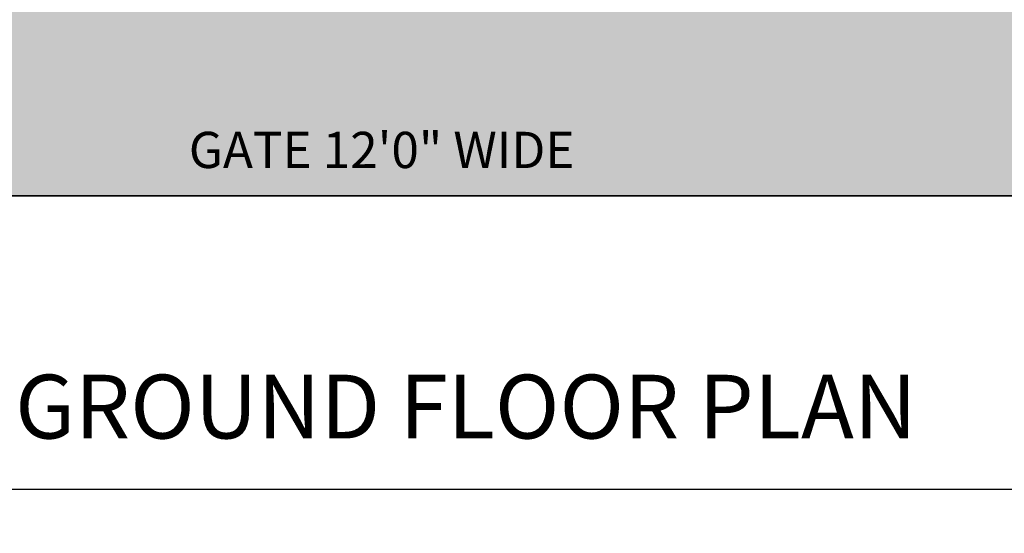
# Model space of a CAD drawing. Units: inches. Extents: x 389 to 971, y 148 to 870.
# Tile 1 of 14: x 448 to 565, y 194 to 256. Entities that reach past the tile are written whole.
import ezdxf

# ---------------------------------------------------------------- set-up
doc = ezdxf.new("R2010")
doc.units = ezdxf.units.IN
doc.header["$MEASUREMENT"] = 0
for name, color, linetype, lineweight in [('A-ANNO-DIMS', 2, 'Continuous', 18), ('A-ANNO-TEXT', 7, 'Continuous', 18), ('A-ANNO-TITL', 7, 'Continuous', 25), ('C-PROP', 7, 'Continuous', 35), ('L-GATE', 4, 'Continuous', 25), ('L-GRND-BASE-PATT', 8, 'Continuous', 13)]:
    doc.layers.add(name, color=color, linetype=linetype, lineweight=lineweight)
doc.layers.add('L-GRND-PATT', color=39, linetype='Continuous', lineweight=13, true_color=0x603913)
doc.styles.get("Standard").update_dxf_attribs({"font": 'arial.ttf'})
doc.dimstyles.get("Standard").update_dxf_attribs({"dimtxt": 8, "dimasz": 8, "dimexe": 0.18, "dimexo": 0.0625, "dimgap": 0.09, "dimtad": 0, "dimtih": 1, "dimtoh": 1, "dimdec": 0, "dimzin": 0, "dimdsep": 46, "dimlunit": 3, "dimtxsty": 'Standard', "dimcen": 0.09, "dimadec": 0, "dimazin": 0, "dimtfac": 1, "dimtdec": 0, "dimtofl": 0, "dimtmove": 0, "dimatfit": 3, "dimfxl": 1, "dimtolj": 1, "dimtzin": 0, "dimarcsym": 0})

# ---------------------------------------------------------------- blocks, each defined once
blk = doc.blocks.new('*D44')
at = {"layer": 'A-ANNO-DIMS', "color": 0, "lineweight": -2, "transparency": 16777216}
for p, q in [((428.216024, 234.582013), (428.216024, 199.495293)), ((848.2160239999998, 234.582013), (848.2160239999998, 199.495293)), ((436.216024, 199.675293), (629.1410308212824, 199.675293)), ((840.2160239999998, 199.675293), (647.2910171787175, 199.675293))]:
    blk.add_line(p, q, dxfattribs=at)
at = {"layer": 'A-ANNO-DIMS', "color": 0, "transparency": 16777216}
for points in [[(436.216024, 201.0086263333334), (436.216024, 198.3419596666666), (428.216024, 199.675293)], [(840.2160239999998, 201.0086263333334), (840.2160239999998, 198.3419596666666), (848.2160239999998, 199.675293)]]:
    blk.add_solid(points, dxfattribs=at)
at = {"layer": 'Defpoints', "color": 0, "transparency": 16777216}
for p in [(428.216024, 234.644513), (848.2160239999998, 234.644513), (848.2160239999998, 199.675293)]:
    blk.add_point(p, dxfattribs=at)
at = {"layer": 'A-ANNO-DIMS', "color": 0, "transparency": 16777216, "insert": (638.216024, 199.675293), "char_height": 8, "attachment_point": 5}
blk.add_mtext('\\A1;420', dxfattribs=at)

msp = doc.modelspace()

# ---------------------------------------------------------------- hatches: boundary and pattern name
at = {"layer": 'L-GRND-BASE-PATT'}
h = msp.add_hatch(color=256, dxfattribs=at)
h.dxf.hatch_style = 1
edge = h.paths.add_edge_path(flags=16)
edge.add_ellipse((8782.002602781105, 354.2472542798386), major_axis=(-8296.949265805946, 5.39345e-11), ratio=0.8423038695428886, start_angle=-0.0902290885933894, end_angle=0.3838667787920258, ccw=False)
edge.add_ellipse((485.0533369751568, 368.2895347624687), major_axis=(-1.159084047334488, 1.838e-13), ratio=0.8423038695439892, start_angle=9.094947017729282e-12, end_angle=90.00000000000898, ccw=False)
edge.add_line((483.8942529278224, 368.2895347624687), (483.8942529278225, 387.6039063360424))
edge.add_ellipse((485.0533369751571, 387.2465553762829), major_axis=(1.159084047334488, 1.838e-13), ratio=0.8423038695439892, start_angle=89.99999999999102, end_angle=179.9999999999909, ccw=False)
edge.add_line((485.0533369751572, 388.2228563544795), (485.5047440247956, 388.2228563544795))
edge.add_ellipse((898.8202485054873, 372.489720535918), major_axis=(413.7373561031672, 1.26113e-11), ratio=0.8423038695441164, start_angle=176.3495724142986, end_angle=177.8200496863524, ccw=False)
edge.add_ellipse((535.9119176052733, 196.3854951855018), major_axis=(-245.3971626940985, 1.013648e-10), ratio=0.8423038695442548, start_angle=-77.87403444769302, end_angle=-76.2194710104792, ccw=False)
edge.add_ellipse((535.9119176052684, 201.7546502845751), major_axis=(239.1273775699096, 1.008988e-10), ratio=0.842303869543627, start_angle=100.20953899711827, end_angle=102.44462729341922, ccw=False)
edge.add_ellipse((473.3138688667988, 564.9222417143382), major_axis=(196.5636751472093, 8.4793e-12), ratio=0.8423038695439335, start_angle=-80.74343399280163, end_angle=-77.44506735586587)
edge.add_line((509.5535496243029, 402.1940957519602), (514.3535105156315, 404.8483349684994))
edge.add_line((514.3535105156315, 404.8483349684994), (514.3535105156315, 404.7971763262221))
edge.add_ellipse((514.3535105156316, 404.2643898676136), major_axis=(0.5795420236673633, 2e-16), ratio=0.8423038695437671, start_angle=52.06686954015339, end_angle=90.00000000001342, ccw=False)
edge.add_line((514.671564037824, 404.672460591463), (519.1534714069603, 402.19409575196))
edge.add_ellipse((555.3931521644682, 564.9222417143374), major_axis=(-196.5636751472384, 3.62381e-11), ratio=0.8423038695438114, start_angle=77.44506735587258, end_angle=80.74343399280833)
edge.add_ellipse((492.795103425985, 201.7546502845724), major_axis=(239.12737756976, 4.82267e-11), ratio=0.8423038695441539, start_angle=77.55537270654253, end_angle=79.7904610028433, ccw=False)
edge.add_ellipse((492.7951034259847, 196.3854951855023), major_axis=(245.3971626940514, 1.422861e-10), ratio=0.8423038695444116, start_angle=76.21947101046823, end_angle=77.87403444768199, ccw=False)
edge.add_ellipse((129.8867725257751, 372.4897205359271), major_axis=(-413.7373561031673, 2.44623e-11), ratio=0.8423038695441432, start_angle=182.179950313648, end_angle=183.6504275857018, ccw=False)
edge.add_line((543.2022770064673, 388.2228563544788), (544.0779382625514, 388.2228563544787))
edge.add_ellipse((543.6536840561057, 387.2465553762822), major_axis=(-1.159084047334545, 1.527e-13), ratio=0.8423038695438989, start_angle=180.0000000000075, end_angle=270.00000000000756, ccw=False)
edge.add_line((544.8127681034401, 387.2465553762826), (544.8127681034399, 367.9321838027083))
edge.add_ellipse((543.6536840561054, 368.2895347624679), major_axis=(1.159084047334544, 7.24e-14), ratio=0.8423038695439478, start_angle=269.9999999999964, end_angle=359.9999999999964, ccw=False)
edge.add_ellipse((-7753.295581726658, 354.2472542799028), major_axis=(-8296.949265782761, 2.068448e-10), ratio=0.8423038695442414, start_angle=179.6161332212083, end_angle=180.0902290885951, ccw=False)
edge.add_line((543.3912265319653, 298.6607849184036), (544.0779382625504, 298.6607849184036))
edge.add_ellipse((543.6536840561046, 297.6844839402071), major_axis=(1.159084047334431, 1.769e-13), ratio=0.8423038695439814, start_angle=-1.1482370609883219e-11, end_angle=89.99999999999119, ccw=False)
edge.add_line((544.8127681034391, 297.684483940207), (544.8127681034387, 278.3701123666333))
edge.add_ellipse((543.6536840561043, 278.727463326393), major_axis=(-1.159084047334431, 2.574e-13), ratio=0.8423038695440306, start_angle=90.00000000001268, end_angle=180.0000000000099, ccw=False)
edge.add_line((543.6536840561045, 277.7511623481965), (543.1566278692261, 277.7511623481965))
edge.add_ellipse((-7753.295581726658, 354.2472542799028), major_axis=(-8296.949265782761, 2.068448e-10), ratio=0.8423038695442414, start_angle=179.3813568036816, end_angle=179.4717285281829, ccw=False)
edge.add_ellipse((542.4236240941387, 263.2762864208561), major_axis=(-1.738626071001761, 2.132e-13), ratio=0.8423038695439151, start_angle=179.3717627838137, end_angle=248.464756601011, ccw=False)
edge.add_ellipse((-7753.875123750511, 354.2472542780016), major_axis=(-8298.740341433751, 2.4782644722e-06), ratio=0.8423038662721074, start_angle=179.3534459200609, end_angle=179.3717628008941, ccw=False)
edge.add_ellipse((540.0116322079951, 260.6509346628677), major_axis=(-4.109243751168186, 2.384e-13), ratio=0.842303869543976, start_angle=90.0000000000635, end_angle=179.3534459029233, ccw=False)
edge.add_line((540.0116322079991, 257.1897027503593), (488.6953888232593, 257.1897027503609))
edge.add_ellipse((488.6953888232669, 260.6509346628715), major_axis=(4.10924375117072, 1.262e-13), ratio=0.8423038695439824, start_angle=180.6465540970565, end_angle=269.9999999998589, ccw=False)
edge.add_ellipse((8782.582144816053, 354.2472542821698), major_axis=(-8298.740341477976, 1.8591886369e-06), ratio=0.8423038720186145, start_angle=0.6282372290784792, end_angle=0.6465541099116194, ccw=False)
edge.add_ellipse((486.2833969371199, 263.2762864208594), major_axis=(-1.738626071002378, 2.7e-13), ratio=0.8423038695439394, start_angle=-68.46475649596817, end_angle=0.6282372161796275, ccw=False)
edge.add_ellipse((8782.002602781105, 354.2472542798386), major_axis=(-8296.949265805946, 5.39345e-11), ratio=0.8423038695428886, start_angle=0.5282714718171064, end_angle=0.6465540970606867, ccw=False)
edge.add_line((485.5503931620382, 277.7511623481972), (484.6290827687102, 277.7511623481972))
edge.add_ellipse((485.0533369751559, 278.7274633263938), major_axis=(-1.159084047334545, 3.11e-13), ratio=0.8423038695439968, start_angle=1.5404566511278972e-11, end_angle=90.000000000012, ccw=False)
edge.add_line((483.8942529278214, 278.7274633263938), (483.8942529278216, 298.0418348999672))
edge.add_ellipse((485.053336975156, 297.6844839402078), major_axis=(1.159084047334488, 1.025e-13), ratio=0.8423038695440382, start_angle=89.99999999999488, end_angle=179.9999999999949, ccw=False)
edge = h.paths.add_edge_path(flags=0)
edge.add_ellipse((8782.002602781096, 354.247254279773), major_axis=(-8295.790181758603, 9.87839e-10), ratio=0.8423038695486498, start_angle=0.05559431350519617, end_angle=0.37776419391582294, ccw=False)
edge.add_line((486.2179253655185, 346.1978202249628), (489.3905023836935, 335.8383575186984))
edge.add_ellipse((3386.011413077446, 329.726312794031), major_axis=(-2896.629999631248, 1.069454e-10), ratio=0.8423038695494893, start_angle=-0.1208973690315206, end_angle=0.3640763488915184)
edge.add_line((489.4638383140943, 311.3204429697198), (486.4665645878948, 299.5520931219791))
edge = h.paths.add_edge_path(flags=0)
edge.add_ellipse((514.3535105156315, 391.3730654902235), major_axis=(-115.1512533244504, 1.8736e-12), ratio=0.8423038695439684, start_angle=76.4018653097696, end_angle=103.5981346902308)
edge.add_line((537.3427693057832, 296.3333211885938), (537.342769305783, 281.5897392316151))
edge.add_ellipse((514.3535105156313, 376.6294835332447), major_axis=(-115.1512533244486, 9.02e-13), ratio=0.8423038695439828, start_angle=76.40186530976922, end_angle=103.59813469023032, ccw=False)
edge.add_line((491.3642517254773, 281.5897392316156), (491.3642517254774, 296.3333211885945))
edge = h.paths.add_edge_path(flags=0)
edge.add_line((491.3642517254777, 337.0752369161334), (489.6529508739416, 349.9015767089268))
edge.add_ellipse((510.1338164488795, 298.7862183048575), major_axis=(64.04807894948699, 3.9006e-12), ratio=0.8423038695439252, start_angle=94.27742096304979, end_angle=111.83495379670401, ccw=False)
edge.add_line((506.106812905481, 352.6274231954524), (522.600208125781, 352.6274231954521))
edge.add_ellipse((518.5732045823798, 298.7862183048586), major_axis=(64.04807894948067, 3.24e-14), ratio=0.8423038695439885, start_angle=68.16504620328948, end_angle=85.72257903694378, ccw=False)
edge.add_line((539.05407015732, 349.9015767089259), (537.3427693057835, 337.0752369161327))
edge.add_ellipse((516.5461636849332, 287.5825181681899), major_axis=(62.33048198262021, 1.5954e-12), ratio=0.8423038695439995, start_angle=67.20808512240782, end_angle=85.12993040286212)
edge.add_line((521.0080028322477, 339.9490379899644), (507.6990181990146, 339.9490379899646))
edge.add_ellipse((512.1608573463288, 287.5825181681774), major_axis=(62.33048198263887, 2.0798e-12), ratio=0.8423038695439498, start_angle=94.8700695971331, end_angle=112.791914877584)
edge = h.paths.add_edge_path(flags=0)
edge.add_ellipse((493.6824198201462, 273.9438556676354), major_axis=(-2.318168094668919, 1.896e-13), ratio=0.8423038695439611, start_angle=-89.99999999999523, end_angle=4.718003765447065e-12, ccw=False)
edge.add_line((493.6824198201462, 275.8964576240284), (535.3743409680425, 275.8964576240277))
edge.add_ellipse((535.024601211114, 273.9438556676347), major_axis=(2.318168094668976, 2.946e-13), ratio=0.8423038695439647, start_angle=-7.275957614183426e-12, end_angle=89.99999999998943, ccw=False)
edge.add_line((537.342769305783, 273.9438556676347), (537.3427693057827, 258.698332706474))
edge.add_line((537.3427693057827, 258.698332706474), (540.5911742316662, 258.6983327064739))
edge.add_ellipse((540.5911742316634, 260.6509346628669), major_axis=(-2.318168094668839, 2.143e-13), ratio=0.8423038695440144, start_angle=90.00000000008203, end_angle=179.3534459029346)
edge.add_line((540.5911742316662, 258.6983327064739), (487.7691399811528, 258.6983327064755))
edge.add_ellipse((488.1158467995968, 260.6509346628684), major_axis=(2.318168094668909, 7.48e-14), ratio=0.8423038695439647, start_angle=180.6465540970884, end_angle=269.9999999999081)
edge.add_line((488.1158467995931, 258.6983327064755), (491.3642517254771, 258.6983327064754))
edge.add_line((491.3642517254771, 258.6983327064754), (491.3642517254771, 274.2384428182294))
h.paths.add_polyline_path([(746.1375687288224, 327.3223047166553), (750.1400147212453, 327.3223047166553), (750.1400147212453, 326.2830696147227), (798.1693712998389, 326.2830696147227), (798.1693712998389, 327.3223047166553), (802.1718172922616, 327.3223047166553), (802.1718172922616, 309.9783792024682, -0.1904762075443491), (746.1375687288224, 309.9783668090107)], flags=16)
h.paths.add_polyline_path([(782.1595875801748, 313.5684994305933), (782.1595893317732, 309.0414930416419, -0.0496282101666581), (766.1497986905329, 309.0414910503953), (766.1498004421323, 313.5684994305933)], flags=0)
h.paths.add_polyline_path([(755.1858908233534, 344.9352232902417), (755.1858908233534, 373.916311072083), (788.1243995226009, 373.916311072083), (788.1243995226009, 344.9352232902417)], flags=16)
h.paths.add_polyline_path([(757.1858908233535, 346.9352232902417), (757.1858908233535, 371.916311072083), (786.1243995226009, 371.916311072083), (786.1243995226009, 346.9352232902417)], flags=0)
h.paths.add_polyline_path([(803.6445810111745, 338.4878931208803), (803.6445810111745, 342.4903391133031), (804.6838161131072, 342.4903391133031), (804.6838161131072, 390.5196956918968), (803.6445810111748, 390.5196956918968), (803.6445810111748, 394.5221416843196), (820.9885065253617, 394.5221416843196, -0.1904762075443491), (820.9885189188192, 338.4878931208803)], flags=16)
h.paths.add_polyline_path([(806.8706930931005, 326.6963103558256), (806.4254411777042, 327.1415622712219), (806.4723791864895, 326.6297175483474)], flags=16)
h.paths.add_polyline_path([(822.0328146004263, 317.4007976138144), (822.1941503181826, 317.8932883068639), (821.562628166435, 317.9885306563034)], flags=16)
h.paths.add_polyline_path([(817.3983862972365, 358.5001248341902), (817.3983862972365, 374.5099119722327), (821.9253926861879, 374.5099137238312, -0.049628210166658), (821.9253946774346, 358.5001230825909)], flags=0)
h.paths.add_polyline_path([(808.1446344648577, 418.9736619306146), (808.2246858861593, 418.5632188717996), (808.5395491501399, 418.5787472453325)], flags=16)
h.paths.add_polyline_path([(820.3158762739024, 412.6690288868844), (820.4772119916585, 413.161519579934), (819.8456898399113, 413.2567619293735)], flags=16)
h.paths.add_polyline_path([(466.3155093563569, 235.5246322146605), (517.3806533266912, 235.5246322146605), (517.3806533266912, 244.4269231682286), (466.3155093563569, 244.4269231682286)], flags=24)
h.paths.add_polyline_path([(739.8737195480014, 256.2000079819968), (815.4040239338423, 256.2000079819968), (815.4040239338423, 265.3453807094367), (739.8737195480014, 265.3453807094367)], flags=24)
h.paths.add_polyline_path([(750.6081538187397, 393.6666679930368), (791.5680640722773, 393.6666679930368), (791.5680640722773, 412.3933175868746), (750.6081538187397, 412.3933175868746)], flags=24)
h.paths.add_polyline_path([(438.9630812812552, 410.0618566955462), (484.6203810968238, 410.0618566955462), (484.6203810968238, 429.1217352891893), (438.9630812812552, 429.1217352891893)], flags=24)
edge = h.paths.add_edge_path()
edge.add_line((839.2160244416713, 285.6445131961097), (611.8786784019748, 285.6445131961099))
edge.add_line((611.8786784019748, 285.6445131961099), (604.3870116090119, 285.6445131961097))
edge.add_line((604.3870116090119, 285.6445131961097), (595.3870116090119, 285.6445131961097))
edge.add_line((595.3870116090119, 285.6445131961097), (595.3870116090118, 370.1553848722774))
edge.add_line((595.3870116090118, 370.1553848722774), (604.0816928471932, 370.1553848722774))
edge.add_line((604.0816928471932, 370.1553848722774), (604.0816928471932, 371.3788335667469))
edge.add_line((604.0816928471932, 371.3788335667469), (632.0194586761203, 371.3788335667469))
edge.add_arc((604.0816928471932, 370.1553848722773), 27.96454158787471, 2.507490703587644, 90.00000000000003)
edge.add_line((604.0816928471932, 398.1199264601519), (599.8870116090108, 398.1652144688576))
edge.add_line((599.8870116090108, 398.1652144688576), (604.4225424425357, 398.1652144688576))
edge.add_arc((604.4225424425357, 428.4020866923496), 30.23687222349201, 270.0000000000002, 357.492509296413)
edge.add_line((634.6304631740308, 427.0792235325719), (604.4225424425357, 427.0792235325719))
edge.add_line((604.4225424425357, 427.0792235325719), (604.4225424425357, 428.4020866923497))
edge.add_line((604.4225424425357, 428.4020866923497), (599.8870116090119, 428.4020866923497))
edge.add_line((599.8870116090119, 428.4020866923497), (595.3870116090116, 428.4020866923497))
edge.add_line((595.3870116090116, 428.4020866923497), (595.3870116090118, 434.6445131961097))
edge.add_line((595.3870116090118, 434.6445131961097), (585.0790669792458, 434.6445131961097))
edge.add_line((585.0790669792458, 434.6445131961097), (540.3921730610418, 434.6445131961097))
edge.add_line((540.3921730610418, 434.6445131961097), (526.712508448134, 434.6445131961097))
edge.add_line((526.712508448134, 434.6445131961097), (488.4094553949635, 434.6445131961097))
edge.add_line((488.4094553949635, 434.6445131961097), (432.2160244416713, 434.6445131961097))
edge.add_line((432.2160244416713, 434.6445131961097), (432.2160244416713, 243.6445131961098))
edge.add_line((432.2160244416713, 243.6445131961098), (437.2160244416714, 243.6445131961098))
edge.add_line((437.2160244416714, 243.6445131961098), (437.2160244416714, 234.6445131961098))
edge.add_line((437.2160244416714, 234.6445131961098), (581.2160244416713, 234.6445131961098))
edge.add_line((581.2160244416713, 234.6445131961098), (581.2160244416713, 238.6445131961097))
edge.add_line((581.2160244416713, 238.6445131961097), (581.2160244416713, 243.6445131961098))
edge.add_line((581.2160244416713, 243.6445131961098), (590.2160244416713, 243.6445131961098))
edge.add_line((590.2160244416713, 243.6445131961098), (590.2160244416713, 238.6445131961097))
edge.add_line((590.2160244416713, 238.6445131961097), (839.2160244416713, 238.6445131961098))
edge.add_line((839.2160244416713, 238.6445131961098), (839.2160244416713, 285.6445131961097))
at = {"layer": 'L-GRND-PATT'}
h = msp.add_hatch(dxfattribs=at)
h.set_pattern_fill('EARTH', color=256, angle=45)
h.set_pattern_definition([(45, (0, 0), (0, 8.980256121069154), [6.349999999999999, -6.349999999999999]), (45, (-1.683798022700466, 1.683798022700466), (0, 8.980256121069154), [6.349999999999999, -6.349999999999999]), (45, (-3.367596045400933, 3.367596045400933), (0, 8.980256121069154), [6.349999999999999, -6.349999999999999]), (135, (-3.367596045400933, 4.490128060534576), (-8.980256121069154, 0), [6.349999999999999, -6.349999999999999]), (135, (-1.683798022700466, 6.173926083235043), (-8.980256121069154, 0), [6.349999999999999, -6.349999999999999]), (135, (0, 7.85772410593551), (-8.980256121069154, 0), [6.349999999999999, -6.349999999999999])])
h.paths.add_polyline_path([(432.2160244416713, 243.6445131961098), (437.2160244416714, 243.6445131961098), (437.2160244416714, 234.6445131961098), (581.2160244416713, 234.6445131961098), (581.2160244416713, 238.6445131961097), (581.2160244416713, 243.6445131961098), (590.2160244416713, 243.6445131961098), (590.2160244416713, 238.6445131961097), (839.2160244416713, 238.6445131961098), (839.2160244416712, 285.6445131961097), (810.0513609197296, 285.6445131961097), (733.8056934525983, 285.6445131961099), (684.2433676403508, 285.6445131961098), (611.8786784019748, 285.6445131961099), (604.3870116090119, 285.6445131961097), (595.3870116090119, 285.6445131961097), (595.3870116090118, 370.1553848722774), (604.0816928471932, 370.1553848722774), (604.0816928471932, 371.3788335667469), (632.0194586761203, 371.3788335667469, 0.4014527144963568), (604.0816928471932, 398.119926460152), (599.8870116090127, 398.1652144688576), (604.4225424425357, 398.1652144688576, 0.4014527144963579), (634.6304631740308, 427.0792235325719), (604.4225424425357, 427.0792235325719), (604.4225424425357, 428.4020866923497), (599.8870116090119, 428.4020866923497), (595.3870116090116, 428.4020866923497), (595.3870116090118, 434.6445131961097), (585.0790669792458, 434.6445131961097), (540.3921730610418, 434.6445131961097), (526.712508448134, 434.6445131961097), (488.4094553949635, 434.6445131961097), (432.2160244416713, 434.6445131961097)])
edge = h.paths.add_edge_path(flags=16)
edge.add_line((483.8942529278214, 278.7274633263938), (483.8942529278216, 298.2563878122772))
edge.add_ellipse((485.053336975156, 297.6844839402078), major_axis=(1.159084047334488, 1.025e-13), ratio=0.8423038695440382, start_angle=89.99999999999488, end_angle=179.9999999999949, ccw=False)
edge.add_ellipse((8782.002602781105, 354.2472542798386), major_axis=(-8296.949265805946, 5.39345e-11), ratio=0.8423038695428886, start_angle=-0.0902290885933894, end_angle=0.3838667787920258, ccw=False)
edge.add_ellipse((485.0533369751568, 368.2895347624687), major_axis=(-1.159084047334488, 1.838e-13), ratio=0.8423038695439892, start_angle=9.094947017729282e-12, end_angle=90.00000000000898, ccw=False)
edge.add_line((483.8942529278224, 368.2895347624687), (483.8942529278225, 387.8184592483523))
edge.add_ellipse((485.0533369751571, 387.2465553762829), major_axis=(1.159084047334488, 1.838e-13), ratio=0.8423038695439892, start_angle=89.99999999999102, end_angle=179.9999999999909, ccw=False)
edge.add_ellipse((898.8202485054873, 372.489720535918), major_axis=(413.7373561031672, 1.26113e-11), ratio=0.8423038695441164, start_angle=176.3495724142986, end_angle=177.8200496863524, ccw=False)
edge.add_ellipse((535.9119176052733, 196.3854951855018), major_axis=(-245.3971626940985, 1.013648e-10), ratio=0.8423038695442548, start_angle=-77.87403444769302, end_angle=-76.2194710104792, ccw=False)
edge.add_ellipse((535.9119176052684, 201.7546502845751), major_axis=(239.1273775699096, 1.008988e-10), ratio=0.842303869543627, start_angle=100.20953899711827, end_angle=102.44462729341922, ccw=False)
edge.add_ellipse((473.3138688667988, 564.9222417143382), major_axis=(196.5636751472093, 8.4793e-12), ratio=0.8423038695439335, start_angle=-80.74343399280163, end_angle=-77.44506735586587)
edge.add_line((509.5535496243029, 402.1940957519602), (514.3535105156316, 404.8483349684994))
edge.add_line((514.3535105156316, 404.8483349684994), (519.1534714069603, 402.19409575196))
edge.add_ellipse((555.3931521644682, 564.9222417143374), major_axis=(-196.5636751472384, 3.62381e-11), ratio=0.8423038695438114, start_angle=77.44506735587258, end_angle=80.74343399280833)
edge.add_ellipse((492.795103425985, 201.7546502845724), major_axis=(239.12737756976, 4.82267e-11), ratio=0.8423038695441539, start_angle=77.55537270654253, end_angle=79.7904610028433, ccw=False)
edge.add_ellipse((492.7951034259847, 196.3854951855023), major_axis=(245.3971626940514, 1.422861e-10), ratio=0.8423038695444116, start_angle=76.21947101046823, end_angle=77.87403444768199, ccw=False)
edge.add_ellipse((129.8867725257751, 372.4897205359271), major_axis=(-413.7373561031673, 2.44623e-11), ratio=0.8423038695441432, start_angle=182.179950313648, end_angle=183.6504275857018, ccw=False)
edge.add_line((543.2022770064673, 388.2228563544789), (544.3326597711041, 388.2228563544786))
edge.add_ellipse((543.6536840561057, 387.2465553762822), major_axis=(-1.159084047334545, 1.527e-13), ratio=0.8423038695438989, start_angle=180.0000000000075, end_angle=270.00000000000756, ccw=False)
edge.add_line((544.8127681034401, 387.2465553762825), (544.8127681034399, 367.7176308903986))
edge.add_ellipse((543.6536840561054, 368.2895347624679), major_axis=(1.159084047334544, 7.24e-14), ratio=0.8423038695439478, start_angle=269.9999999999964, end_angle=359.9999999999964, ccw=False)
edge.add_ellipse((-7753.295581726658, 354.2472542799028), major_axis=(-8296.949265782761, 2.068448e-10), ratio=0.8423038695442414, start_angle=179.6161332212083, end_angle=180.0902290885951, ccw=False)
edge.add_ellipse((543.6536840561046, 297.6844839402071), major_axis=(1.159084047334431, 1.769e-13), ratio=0.8423038695439814, start_angle=-1.1482370609883219e-11, end_angle=89.99999999999119, ccw=False)
edge.add_line((544.8127681034391, 297.6844839402071), (544.8127681034387, 278.1555594543235))
edge.add_ellipse((543.6536840561043, 278.727463326393), major_axis=(-1.159084047334431, 2.574e-13), ratio=0.8423038695440306, start_angle=90.00000000001268, end_angle=180.0000000000099, ccw=False)
edge.add_ellipse((-7753.295581726658, 354.2472542799028), major_axis=(-8296.949265782761, 2.068448e-10), ratio=0.8423038695442414, start_angle=179.3813568036816, end_angle=179.4717285281829, ccw=False)
edge.add_ellipse((542.4236240941387, 263.2762864208561), major_axis=(-1.738626071001761, 2.132e-13), ratio=0.8423038695439151, start_angle=179.3717627838137, end_angle=248.464756601011, ccw=False)
edge.add_ellipse((-7753.875123750511, 354.2472542780016), major_axis=(-8298.740341433751, 2.4782644722e-06), ratio=0.8423038662721074, start_angle=179.3534459200609, end_angle=179.3717628008941, ccw=False)
edge.add_ellipse((540.0116322079951, 260.6509346628677), major_axis=(-4.109243751168186, 2.384e-13), ratio=0.842303869543976, start_angle=90.0000000000635, end_angle=179.3534459029233, ccw=False)
edge.add_line((540.0116322079989, 257.1897027503593), (488.0808074948215, 257.1897027503609))
edge.add_ellipse((488.6953888232669, 260.6509346628715), major_axis=(4.10924375117072, 1.262e-13), ratio=0.8423038695439824, start_angle=180.6465540970565, end_angle=269.9999999998589, ccw=False)
edge.add_ellipse((8782.582144816053, 354.2472542821698), major_axis=(-8298.740341477976, 1.8591886369e-06), ratio=0.8423038720186145, start_angle=0.6282372290784792, end_angle=0.6465541099116194, ccw=False)
edge.add_ellipse((486.2833969371199, 263.2762864208594), major_axis=(-1.738626071002378, 2.7e-13), ratio=0.8423038695439394, start_angle=-68.46475649596817, end_angle=0.6282372161796275, ccw=False)
edge.add_ellipse((8782.002602781105, 354.2472542798386), major_axis=(-8296.949265805946, 5.39345e-11), ratio=0.8423038695428886, start_angle=0.5282714718171064, end_angle=0.6465540970606867, ccw=False)
edge.add_line((485.5503931620382, 277.7511623481972), (484.3743612601578, 277.7511623481972))
edge.add_ellipse((485.0533369751559, 278.7274633263938), major_axis=(-1.159084047334545, 3.11e-13), ratio=0.8423038695439968, start_angle=1.5404566511278972e-11, end_angle=90.000000000012, ccw=False)
edge = h.paths.add_edge_path(flags=0)
edge.add_ellipse((488.1158467995968, 260.6509346628684), major_axis=(2.318168094668909, 7.48e-14), ratio=0.8423038695439647, start_angle=180.6465540970884, end_angle=269.9999999999081)
edge.add_line((488.1158467995933, 258.6983327064755), (491.3642517254771, 258.6983327064753))
edge.add_line((491.3642517254771, 258.6983327064753), (491.3642517254771, 274.4686391213292))
edge.add_ellipse((493.6824198201462, 273.9438556676354), major_axis=(-2.318168094668919, 1.896e-13), ratio=0.8423038695439611, start_angle=-89.99999999999523, end_angle=4.718003765447065e-12, ccw=False)
edge.add_line((493.6824198201462, 275.8964576240284), (535.6476346230087, 275.8964576240277))
edge.add_ellipse((535.024601211114, 273.9438556676347), major_axis=(2.318168094668976, 2.946e-13), ratio=0.8423038695439647, start_angle=-7.275957614183426e-12, end_angle=89.99999999998943, ccw=False)
edge.add_line((537.342769305783, 273.9438556676347), (537.3427693057827, 258.698332706474))
edge.add_line((537.3427693057827, 258.698332706474), (541.2086129152347, 258.6983327064739))
edge.add_ellipse((540.5911742316634, 260.6509346628669), major_axis=(-2.318168094668839, 2.143e-13), ratio=0.8423038695440144, start_angle=90.00000000008203, end_angle=179.3534459029347, ccw=False)
edge.add_line((540.5911742316662, 258.6983327064739), (487.4984081160257, 258.6983327064755))
edge = h.paths.add_edge_path(flags=0)
edge.add_line((491.3642517254773, 281.5897392316156), (491.3642517254774, 296.3333211885945))
edge.add_ellipse((514.3535105156315, 391.3730654902235), major_axis=(-115.1512533244504, 1.8736e-12), ratio=0.8423038695439684, start_angle=76.4018653097696, end_angle=103.5981346902308)
edge.add_line((537.3427693057832, 296.3333211885938), (537.342769305783, 281.5897392316151))
edge.add_ellipse((514.3535105156313, 376.6294835332447), major_axis=(-115.1512533244486, 9.02e-13), ratio=0.8423038695439828, start_angle=76.40186530976922, end_angle=103.59813469023032, ccw=False)
edge = h.paths.add_edge_path(flags=0)
edge.add_ellipse((8782.002602781096, 354.247254279773), major_axis=(-8295.790181758603, 9.87839e-10), ratio=0.8423038695486498, start_angle=0.05559431350519617, end_angle=0.37776419391582294, ccw=False)
edge.add_line((486.2179253655185, 346.1978202249628), (489.3905023836935, 335.8383575186985))
edge.add_ellipse((3386.011413077446, 329.726312794031), major_axis=(-2896.629999631248, 1.069454e-10), ratio=0.8423038695494893, start_angle=-0.1208973690315206, end_angle=0.3640763488915184)
edge.add_line((489.4638383140943, 311.3204429697198), (486.4665645878948, 299.5520931219782))
edge = h.paths.add_edge_path(flags=0)
edge.add_line((491.3642517254777, 337.0752369161334), (489.6529508739416, 349.9015767089268))
edge.add_ellipse((510.1338164488795, 298.7862183048575), major_axis=(64.04807894948699, 3.9006e-12), ratio=0.8423038695439252, start_angle=94.27742096304979, end_angle=111.83495379670401, ccw=False)
edge.add_line((506.106812905481, 352.6274231954524), (522.600208125781, 352.6274231954521))
edge.add_ellipse((518.5732045823798, 298.7862183048586), major_axis=(64.04807894948067, 3.24e-14), ratio=0.8423038695439885, start_angle=68.16504620328948, end_angle=85.72257903694378, ccw=False)
edge.add_line((539.05407015732, 349.9015767089259), (537.3427693057835, 337.0752369161327))
edge.add_ellipse((516.5461636849332, 287.5825181681899), major_axis=(62.33048198262021, 1.5954e-12), ratio=0.8423038695439995, start_angle=67.20808512240782, end_angle=85.12993040286212)
edge.add_line((521.0080028322477, 339.9490379899644), (507.6990181990145, 339.9490379899646))
edge.add_ellipse((512.1608573463288, 287.5825181681774), major_axis=(62.33048198263887, 2.0798e-12), ratio=0.8423038695439498, start_angle=94.8700695971331, end_angle=112.791914877584)
h.paths.add_polyline_path([(466.3155093563569, 235.5246322146605), (517.3806533266912, 235.5246322146605), (517.3806533266912, 244.4269231682286), (466.3155093563569, 244.4269231682286)], flags=24)
h.paths.add_polyline_path([(739.8737195480014, 256.2000079819968), (815.4040239338423, 256.2000079819968), (815.4040239338423, 265.3453807094367), (739.8737195480014, 265.3453807094367)], flags=24)
h.paths.add_polyline_path([(438.9630812812552, 410.0618566955462), (484.6203810968238, 410.0618566955462), (484.6203810968238, 429.1217352891893), (438.9630812812552, 429.1217352891893)], flags=24)

# ---------------------------------------------------------------- linework, layer by layer
at = {"layer": 'C-PROP'}
msp.add_line((428.2160244416713, 234.6445131961098), (848.2160244416714, 234.6445131961098), dxfattribs=at)
at = {"layer": 'L-GATE'}
msp.add_line((437.2160244416714, 234.6445131961098), (581.2160244416713, 234.6445131961098), dxfattribs=at)

# ---------------------------------------------------------------- texts
at = {"layer": 'A-ANNO-TEXT', "insert": (467.7167140397139, 242.2772305993349), "char_height": 4.320012756680132, "attachment_point": 1}
msp.add_mtext_dynamic_manual_height_columns('GATE 12\'0" WIDE', width=98.04586917418564, gutter_width=21.60006378340066, heights=[0], dxfattribs=at)
at = {"layer": 'A-ANNO-TITL', "insert": (444.6931758821642, 213.3239792349412), "char_height": 7.597517507942846, "attachment_point": 1}
msp.add_mtext_dynamic_manual_height_columns(' GROUND FLOOR PLAN', width=172.4312518476909, gutter_width=37.98758753971423, heights=[0], dxfattribs=at)

# ---------------------------------------------------------------- dimensions: what is measured, and where the dimension line sits
at = {"layer": 'A-ANNO-DIMS'}
dim = msp.add_linear_dim(base=(848.2160239999998, 199.675293), p1=(428.216024, 234.644513), p2=(848.2160239999998, 234.644513), dimstyle='Standard', override={"dimdec": 0, "dimlfac": 1, "dimrnd": 0, "dimzin": 0, "dimdsep": 46, "dimlunit": 2}, dxfattribs=at)
dim.commit()
dim.dimension.update_dxf_attribs({"geometry": '*D44', "text_midpoint": (638.216024, 199.675293)})

doc.saveas('drawing.dxf')
